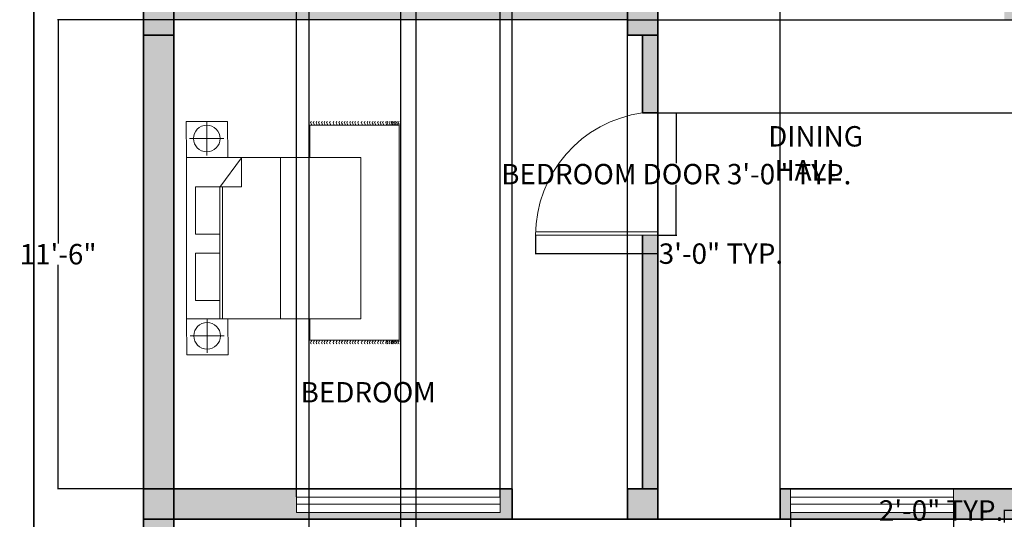
# Model space of a CAD drawing. Units: inches. Extents: x 74 to 548, y 68 to 649.
# Tile 2 of 6: x 79 to 368, y 214 to 361. Entities that reach past the tile are written whole.
import ezdxf

# ---------------------------------------------------------------- set-up
doc = ezdxf.new("R2010")
doc.units = ezdxf.units.IN
doc.header["$MEASUREMENT"] = 0
for name, color, linetype, lineweight in [('A-ANNO-DIMS', 2, 'Continuous', 18), ('A-ANNO-TTLB', 7, 'Continuous', 35), ('A-AREA-IDEN', 7, 'Continuous', 25), ('A-COLS', 7, 'Continuous', 35), ('A-DOOR', 3, 'Continuous', 18), ('A-FURN', 8, 'Continuous', 18), ('A-GLAZ', 4, 'Continuous', 18), ('A-WALL', 7, 'Continuous', 35)]:
    doc.layers.add(name, color=color, linetype=linetype, lineweight=lineweight)
doc.layers.add('A-COLS-PATT', color=11, linetype='Continuous', lineweight=13, true_color=0xf27172)
doc.layers.add('A-WALL-PATT', color=7, linetype='Continuous', lineweight=13, true_color=0xffffff)
doc.styles.get("Standard").update_dxf_attribs({"font": 'arial.ttf'})
doc.dimstyles.get("Standard").update_dxf_attribs({"dimtxt": 6, "dimasz": 0.18, "dimexe": 0.18, "dimexo": 0.0625, "dimgap": 0.09, "dimtad": 0, "dimtih": 1, "dimtoh": 1, "dimdec": 1, "dimzin": 0, "dimdsep": 46, "dimlunit": 3, "dimtxsty": 'Standard', "dimcen": 0.09, "dimadec": 0, "dimazin": 0, "dimtfac": 1, "dimtdec": 1, "dimtofl": 0, "dimtmove": 0, "dimatfit": 3, "dimfxl": 1, "dimtolj": 1, "dimtzin": 0, "dimarcsym": 0})

# ---------------------------------------------------------------- blocks, each defined once
blk = doc.blocks.new('BED-DOUBLE-NIGHTSTANDS')
for p, q in [((-5.03, -1.07), (-5.03, -11.12)), ((53.03, -0.96), (53.03, -11.02)), ((0, -6.09), (-10.05, -6.09)), ((58.05, -5.99), (48, -5.99)), ((38.76, -9.86), (0, -9.86)), ((38.82, -10.68), (0, -10.68)), ((38.76, -9.86), (47.38, -16.22)), ((38.82, -9.86), (38.82, -16.22)), ((38.82, -16.22), (47.38, -16.22)), ((47.43, -27.72), (0, -27.72)), ((-6.27, -62.68), (-6.27, -36.31)), ((-6.27, -36.31), (0.03, -36.31)), ((47.43, -36.31), (56.97, -36.31)), ((56.97, -36.31), (56.97, -62.68)), ((56.97, -62.68), (-6.27, -62.68))]:
    blk.add_line(p, q)
for points in [[(-10.63, -12.29), (0, -12.19), (0, 0), (-10.63, -0.1)], [(47.43, 0), (47.43, -51.32), (0, -51.32), (0, 0)], [(47.43, -12.19), (58.05, -12.08), (58.05, 0.1), (47.43, 0)], [(19.25, -2.7), (19.25, -9.86), (5.36, -9.86), (5.36, -2.7)], [(38.82, -2.7), (38.82, -9.86), (24.92, -9.86), (24.92, -2.7)]]:
    blk.add_lwpolyline(points, close=True)
for centre in [(-5.03, -6.09), (53.03, -5.99)]:
    blk.add_circle(centre, 3.92)
for points, knots in [([(-7.4, -36.85), (-7.3, -36.72), (-7.11, -36.49), (-6.77, -36.72), (-6.49, -36.9), (-6.34, -36.79), (-6.27, -36.74)], [0, 0, 0, 0, 0.400747, 0.791423, 1.067667, 1.29709, 1.29709, 1.29709, 1.29709]), ([(-7.4, -37.62), (-7.3, -37.5), (-7.11, -37.26), (-6.77, -37.5), (-6.49, -37.68), (-6.34, -37.57), (-6.27, -37.52)], [0, 0, 0, 0, 0.400747, 0.791423, 1.067667, 1.29709, 1.29709, 1.29709, 1.29709]), ([(58.08, -36.85), (57.99, -36.72), (57.8, -36.49), (57.45, -36.72), (57.17, -36.9), (57.02, -36.79), (56.96, -36.74)], [0, 0, 0, 0, 0.400747, 0.791423, 1.067667, 1.29709, 1.29709, 1.29709, 1.29709]), ([(58.08, -37.62), (57.99, -37.5), (57.8, -37.26), (57.45, -37.5), (57.17, -37.68), (57.02, -37.57), (56.96, -37.52)], [0, 0, 0, 0, 0.400747, 0.791423, 1.067667, 1.29709, 1.29709, 1.29709, 1.29709]), ([(-7.4, -38.44), (-7.3, -38.32), (-7.11, -38.08), (-6.77, -38.32), (-6.49, -38.49), (-6.34, -38.39), (-6.27, -38.34)], [0, 0, 0, 0, 0.400747, 0.791423, 1.067667, 1.29709, 1.29709, 1.29709, 1.29709]), ([(-7.4, -39.17), (-7.3, -39.05), (-7.11, -38.81), (-6.77, -39.05), (-6.49, -39.22), (-6.34, -39.11), (-6.27, -39.07)], [0, 0, 0, 0, 0.400747, 0.791423, 1.067667, 1.29709, 1.29709, 1.29709, 1.29709]), ([(-7.4, -40.05), (-7.3, -39.93), (-7.11, -39.69), (-6.77, -39.93), (-6.49, -40.1), (-6.34, -40), (-6.27, -39.95)], [0, 0, 0, 0, 0.400747, 0.791423, 1.067667, 1.29709, 1.29709, 1.29709, 1.29709]), ([(-7.4, -40.8), (-7.3, -40.68), (-7.11, -40.44), (-6.77, -40.68), (-6.49, -40.85), (-6.34, -40.75), (-6.27, -40.7)], [0, 0, 0, 0, 0.400747, 0.791423, 1.067667, 1.29709, 1.29709, 1.29709, 1.29709]), ([(58.08, -38.44), (57.99, -38.32), (57.8, -38.08), (57.45, -38.32), (57.17, -38.49), (57.02, -38.39), (56.96, -38.34)], [0, 0, 0, 0, 0.400747, 0.791423, 1.067667, 1.29709, 1.29709, 1.29709, 1.29709]), ([(58.08, -39.17), (57.99, -39.05), (57.8, -38.81), (57.45, -39.05), (57.17, -39.22), (57.02, -39.11), (56.96, -39.07)], [0, 0, 0, 0, 0.400747, 0.791423, 1.067667, 1.29709, 1.29709, 1.29709, 1.29709]), ([(58.08, -40.05), (57.99, -39.93), (57.8, -39.69), (57.45, -39.93), (57.17, -40.1), (57.02, -40), (56.96, -39.95)], [0, 0, 0, 0, 0.400747, 0.791423, 1.067667, 1.29709, 1.29709, 1.29709, 1.29709]), ([(58.08, -40.8), (57.99, -40.68), (57.8, -40.44), (57.45, -40.68), (57.17, -40.85), (57.02, -40.75), (56.96, -40.7)], [0, 0, 0, 0, 0.400747, 0.791423, 1.067667, 1.29709, 1.29709, 1.29709, 1.29709]), ([(-7.4, -41.53), (-7.3, -41.41), (-7.11, -41.17), (-6.77, -41.41), (-6.49, -41.58), (-6.34, -41.48), (-6.27, -41.43)], [0, 0, 0, 0, 0.400747, 0.791423, 1.067667, 1.29709, 1.29709, 1.29709, 1.29709]), ([(-7.4, -42.41), (-7.3, -42.29), (-7.11, -42.05), (-6.77, -42.29), (-6.49, -42.46), (-6.34, -42.36), (-6.27, -42.31)], [0, 0, 0, 0, 0.400747, 0.791423, 1.067667, 1.29709, 1.29709, 1.29709, 1.29709]), ([(-7.4, -43.45), (-7.3, -43.33), (-7.11, -43.09), (-6.77, -43.33), (-6.49, -43.5), (-6.34, -43.39), (-6.27, -43.35)], [0, 0, 0, 0, 0.400747, 0.791423, 1.067667, 1.29709, 1.29709, 1.29709, 1.29709]), ([(58.08, -41.53), (57.99, -41.41), (57.8, -41.17), (57.45, -41.41), (57.17, -41.58), (57.02, -41.48), (56.96, -41.43)], [0, 0, 0, 0, 0.400747, 0.791423, 1.067667, 1.29709, 1.29709, 1.29709, 1.29709]), ([(58.08, -42.41), (57.99, -42.29), (57.8, -42.05), (57.45, -42.29), (57.17, -42.46), (57.02, -42.36), (56.96, -42.31)], [0, 0, 0, 0, 0.400747, 0.791423, 1.067667, 1.29709, 1.29709, 1.29709, 1.29709]), ([(58.08, -43.45), (57.99, -43.33), (57.8, -43.09), (57.45, -43.33), (57.17, -43.5), (57.02, -43.39), (56.96, -43.35)], [0, 0, 0, 0, 0.400747, 0.791423, 1.067667, 1.29709, 1.29709, 1.29709, 1.29709]), ([(-7.4, -44.33), (-7.3, -44.21), (-7.11, -43.97), (-6.77, -44.21), (-6.49, -44.38), (-6.34, -44.28), (-6.27, -44.23)], [0, 0, 0, 0, 0.400747, 0.791423, 1.067667, 1.29709, 1.29709, 1.29709, 1.29709]), ([(-7.4, -45.15), (-7.3, -45.03), (-7.11, -44.79), (-6.77, -45.03), (-6.49, -45.2), (-6.34, -45.09), (-6.27, -45.05)], [0, 0, 0, 0, 0.400747, 0.791423, 1.067667, 1.29709, 1.29709, 1.29709, 1.29709]), ([(-7.4, -45.92), (-7.3, -45.8), (-7.11, -45.56), (-6.77, -45.8), (-6.49, -45.98), (-6.34, -45.87), (-6.27, -45.82)], [0, 0, 0, 0, 0.400747, 0.791423, 1.067667, 1.29709, 1.29709, 1.29709, 1.29709]), ([(58.08, -44.33), (57.99, -44.21), (57.8, -43.97), (57.45, -44.21), (57.17, -44.38), (57.02, -44.28), (56.96, -44.23)], [0, 0, 0, 0, 0.400747, 0.791423, 1.067667, 1.29709, 1.29709, 1.29709, 1.29709]), ([(58.08, -45.15), (57.99, -45.03), (57.8, -44.79), (57.45, -45.03), (57.17, -45.2), (57.02, -45.09), (56.96, -45.05)], [0, 0, 0, 0, 0.400747, 0.791423, 1.067667, 1.29709, 1.29709, 1.29709, 1.29709]), ([(58.08, -45.92), (57.99, -45.8), (57.8, -45.56), (57.45, -45.8), (57.17, -45.98), (57.02, -45.87), (56.96, -45.82)], [0, 0, 0, 0, 0.400747, 0.791423, 1.067667, 1.29709, 1.29709, 1.29709, 1.29709]), ([(-7.4, -46.74), (-7.3, -46.62), (-7.11, -46.38), (-6.77, -46.62), (-6.49, -46.79), (-6.34, -46.69), (-6.27, -46.64)], [0, 0, 0, 0, 0.400747, 0.791423, 1.067667, 1.29709, 1.29709, 1.29709, 1.29709]), ([(-7.4, -47.47), (-7.3, -47.35), (-7.11, -47.11), (-6.77, -47.35), (-6.49, -47.52), (-6.34, -47.41), (-6.27, -47.37)], [0, 0, 0, 0, 0.400747, 0.791423, 1.067667, 1.29709, 1.29709, 1.29709, 1.29709]), ([(-7.4, -48.35), (-7.3, -48.23), (-7.11, -47.99), (-6.77, -48.23), (-6.49, -48.4), (-6.34, -48.3), (-6.27, -48.25)], [0, 0, 0, 0, 0.400747, 0.791423, 1.067667, 1.29709, 1.29709, 1.29709, 1.29709]), ([(-7.4, -49.1), (-7.3, -48.98), (-7.11, -48.74), (-6.77, -48.98), (-6.49, -49.15), (-6.34, -49.05), (-6.27, -49)], [0, 0, 0, 0, 0.400747, 0.791423, 1.067667, 1.29709, 1.29709, 1.29709, 1.29709]), ([(58.08, -46.74), (57.99, -46.62), (57.8, -46.38), (57.45, -46.62), (57.17, -46.79), (57.02, -46.69), (56.96, -46.64)], [0, 0, 0, 0, 0.400747, 0.791423, 1.067667, 1.29709, 1.29709, 1.29709, 1.29709]), ([(58.08, -47.47), (57.99, -47.35), (57.8, -47.11), (57.45, -47.35), (57.17, -47.52), (57.02, -47.41), (56.96, -47.37)], [0, 0, 0, 0, 0.400747, 0.791423, 1.067667, 1.29709, 1.29709, 1.29709, 1.29709]), ([(58.08, -48.35), (57.99, -48.23), (57.8, -47.99), (57.45, -48.23), (57.17, -48.4), (57.02, -48.3), (56.96, -48.25)], [0, 0, 0, 0, 0.400747, 0.791423, 1.067667, 1.29709, 1.29709, 1.29709, 1.29709]), ([(58.08, -49.1), (57.99, -48.98), (57.8, -48.74), (57.45, -48.98), (57.17, -49.15), (57.02, -49.05), (56.96, -49)], [0, 0, 0, 0, 0.400747, 0.791423, 1.067667, 1.29709, 1.29709, 1.29709, 1.29709]), ([(-7.4, -49.83), (-7.3, -49.71), (-7.11, -49.47), (-6.77, -49.71), (-6.49, -49.88), (-6.34, -49.78), (-6.27, -49.73)], [0, 0, 0, 0, 0.400747, 0.791423, 1.067667, 1.29709, 1.29709, 1.29709, 1.29709]), ([(-7.4, -50.71), (-7.3, -50.59), (-7.11, -50.35), (-6.77, -50.59), (-6.49, -50.77), (-6.34, -50.66), (-6.27, -50.61)], [0, 0, 0, 0, 0.400747, 0.791423, 1.067667, 1.29709, 1.29709, 1.29709, 1.29709]), ([(-7.4, -51.75), (-7.3, -51.63), (-7.11, -51.39), (-6.77, -51.63), (-6.49, -51.8), (-6.34, -51.7), (-6.27, -51.65)], [0, 0, 0, 0, 0.400747, 0.791423, 1.067667, 1.29709, 1.29709, 1.29709, 1.29709]), ([(58.08, -49.83), (57.99, -49.71), (57.8, -49.47), (57.45, -49.71), (57.17, -49.88), (57.02, -49.78), (56.96, -49.73)], [0, 0, 0, 0, 0.400747, 0.791423, 1.067667, 1.29709, 1.29709, 1.29709, 1.29709]), ([(58.08, -50.71), (57.99, -50.59), (57.8, -50.35), (57.45, -50.59), (57.17, -50.77), (57.02, -50.66), (56.96, -50.61)], [0, 0, 0, 0, 0.400747, 0.791423, 1.067667, 1.29709, 1.29709, 1.29709, 1.29709]), ([(58.08, -51.75), (57.99, -51.63), (57.8, -51.39), (57.45, -51.63), (57.17, -51.8), (57.02, -51.7), (56.96, -51.65)], [0, 0, 0, 0, 0.400747, 0.791423, 1.067667, 1.29709, 1.29709, 1.29709, 1.29709]), ([(-7.4, -52.63), (-7.3, -52.51), (-7.11, -52.27), (-6.77, -52.51), (-6.49, -52.68), (-6.34, -52.58), (-6.27, -52.53)], [0, 0, 0, 0, 0.400747, 0.791423, 1.067667, 1.29709, 1.29709, 1.29709, 1.29709]), ([(-7.4, -53.45), (-7.3, -53.33), (-7.11, -53.09), (-6.77, -53.33), (-6.49, -53.5), (-6.34, -53.39), (-6.27, -53.35)], [0, 0, 0, 0, 0.400747, 0.791423, 1.067667, 1.29709, 1.29709, 1.29709, 1.29709]), ([(-7.4, -54.14), (-7.3, -54.02), (-7.11, -53.78), (-6.77, -54.02), (-6.49, -54.19), (-6.34, -54.08), (-6.27, -54.04)], [0, 0, 0, 0, 0.400747, 0.791423, 1.067667, 1.29709, 1.29709, 1.29709, 1.29709]), ([(-7.4, -54.95), (-7.3, -54.83), (-7.11, -54.59), (-6.77, -54.83), (-6.49, -55.01), (-6.34, -54.9), (-6.27, -54.85)], [0, 0, 0, 0, 0.400747, 0.791423, 1.067667, 1.29709, 1.29709, 1.29709, 1.29709]), ([(58.08, -52.63), (57.99, -52.51), (57.8, -52.27), (57.45, -52.51), (57.17, -52.68), (57.02, -52.58), (56.96, -52.53)], [0, 0, 0, 0, 0.400747, 0.791423, 1.067667, 1.29709, 1.29709, 1.29709, 1.29709]), ([(58.08, -53.45), (57.99, -53.33), (57.8, -53.09), (57.45, -53.33), (57.17, -53.5), (57.02, -53.39), (56.96, -53.35)], [0, 0, 0, 0, 0.400747, 0.791423, 1.067667, 1.29709, 1.29709, 1.29709, 1.29709]), ([(58.08, -54.14), (57.99, -54.02), (57.8, -53.78), (57.45, -54.02), (57.17, -54.19), (57.02, -54.08), (56.96, -54.04)], [0, 0, 0, 0, 0.400747, 0.791423, 1.067667, 1.29709, 1.29709, 1.29709, 1.29709]), ([(58.08, -54.95), (57.99, -54.83), (57.8, -54.59), (57.45, -54.83), (57.17, -55.01), (57.02, -54.9), (56.96, -54.85)], [0, 0, 0, 0, 0.400747, 0.791423, 1.067667, 1.29709, 1.29709, 1.29709, 1.29709]), ([(-7.4, -55.68), (-7.3, -55.56), (-7.11, -55.32), (-6.77, -55.56), (-6.49, -55.73), (-6.34, -55.63), (-6.27, -55.58)], [0, 0, 0, 0, 0.400747, 0.791423, 1.067667, 1.29709, 1.29709, 1.29709, 1.29709]), ([(-7.4, -56.56), (-7.3, -56.44), (-7.11, -56.2), (-6.77, -56.44), (-6.49, -56.62), (-6.34, -56.51), (-6.27, -56.46)], [0, 0, 0, 0, 0.400747, 0.791423, 1.067667, 1.29709, 1.29709, 1.29709, 1.29709]), ([(-7.4, -57.32), (-7.3, -57.2), (-7.11, -56.96), (-6.77, -57.2), (-6.49, -57.37), (-6.34, -57.26), (-6.27, -57.21)], [0, 0, 0, 0, 0.400747, 0.791423, 1.067667, 1.29709, 1.29709, 1.29709, 1.29709]), ([(-7.4, -58.04), (-7.3, -57.92), (-7.11, -57.68), (-6.77, -57.92), (-6.49, -58.1), (-6.34, -57.99), (-6.27, -57.94)], [0, 0, 0, 0, 0.400747, 0.791423, 1.067667, 1.29709, 1.29709, 1.29709, 1.29709]), ([(58.08, -55.68), (57.99, -55.56), (57.8, -55.32), (57.45, -55.56), (57.17, -55.73), (57.02, -55.63), (56.96, -55.58)], [0, 0, 0, 0, 0.400747, 0.791423, 1.067667, 1.29709, 1.29709, 1.29709, 1.29709]), ([(58.08, -56.56), (57.99, -56.44), (57.8, -56.2), (57.45, -56.44), (57.17, -56.62), (57.02, -56.51), (56.96, -56.46)], [0, 0, 0, 0, 0.400747, 0.791423, 1.067667, 1.29709, 1.29709, 1.29709, 1.29709]), ([(58.08, -57.32), (57.99, -57.2), (57.8, -56.96), (57.45, -57.2), (57.17, -57.37), (57.02, -57.26), (56.96, -57.21)], [0, 0, 0, 0, 0.400747, 0.791423, 1.067667, 1.29709, 1.29709, 1.29709, 1.29709]), ([(58.08, -58.04), (57.99, -57.92), (57.8, -57.68), (57.45, -57.92), (57.18, -58.09), (57.03, -57.99), (56.97, -57.95)], [0, 0, 0, 0, 0.400747, 0.791423, 1.067667, 1.283686, 1.283686, 1.283686, 1.283686]), ([(-7.4, -58.93), (-7.3, -58.81), (-7.11, -58.57), (-6.77, -58.81), (-6.49, -58.98), (-6.34, -58.87), (-6.27, -58.82)], [0, 0, 0, 0, 0.400747, 0.791423, 1.067667, 1.29709, 1.29709, 1.29709, 1.29709]), ([(-7.4, -59.36), (-7.3, -59.23), (-7.11, -58.98), (-6.77, -59.24), (-6.49, -59.41), (-6.34, -59.3), (-6.27, -59.25)], [0, 0, 0, 0, 0.407265, 0.802015, 1.07826, 1.307683, 1.307683, 1.307683, 1.307683]), ([(-7.4, -59.92), (-7.3, -59.8), (-7.11, -59.56), (-6.77, -59.8), (-6.49, -59.97), (-6.34, -59.87), (-6.27, -59.82)], [0, 0, 0, 0, 0.400747, 0.791423, 1.067667, 1.29709, 1.29709, 1.29709, 1.29709]), ([(-7.4, -60.5), (-7.3, -60.38), (-7.11, -60.14), (-6.77, -60.38), (-6.49, -60.55), (-6.34, -60.44), (-6.27, -60.39)], [0, 0, 0, 0, 0.400747, 0.791423, 1.067667, 1.29709, 1.29709, 1.29709, 1.29709]), ([(-7.4, -60.81), (-7.3, -60.68), (-7.11, -60.44), (-6.77, -60.68), (-6.49, -60.86), (-6.34, -60.75), (-6.27, -60.7)], [0, 0, 0, 0, 0.400747, 0.791423, 1.067667, 1.29709, 1.29709, 1.29709, 1.29709]), ([(58.08, -58.93), (57.99, -58.81), (57.8, -58.57), (57.45, -58.81), (57.18, -58.98), (57.03, -58.88), (56.97, -58.83)], [0, 0, 0, 0, 0.400747, 0.791423, 1.067667, 1.283686, 1.283686, 1.283686, 1.283686]), ([(58.08, -59.36), (57.99, -59.23), (57.8, -58.99), (57.45, -59.24), (57.18, -59.41), (57.03, -59.31), (56.97, -59.26)], [0, 0, 0, 0, 0.402903, 0.794912, 1.071156, 1.287177, 1.287177, 1.287177, 1.287177]), ([(58.08, -59.95), (57.99, -59.83), (57.8, -59.59), (57.45, -59.83), (57.18, -60), (57.03, -59.9), (56.97, -59.86)], [0, 0, 0, 0, 0.400747, 0.791423, 1.067667, 1.283686, 1.283686, 1.283686, 1.283686]), ([(58.08, -60.52), (57.99, -60.4), (57.8, -60.16), (57.45, -60.4), (57.18, -60.57), (57.03, -60.47), (56.97, -60.43)], [0, 0, 0, 0, 0.400747, 0.791423, 1.067667, 1.283686, 1.283686, 1.283686, 1.283686]), ([(58.08, -60.83), (57.99, -60.71), (57.8, -60.47), (57.45, -60.71), (57.18, -60.88), (57.03, -60.78), (56.97, -60.74)], [0, 0, 0, 0, 0.400747, 0.791423, 1.067667, 1.283686, 1.283686, 1.283686, 1.283686]), ([(-7.4, -61.22), (-7.3, -61.1), (-7.11, -60.86), (-6.77, -61.1), (-6.49, -61.28), (-6.34, -61.17), (-6.27, -61.12)], [0, 0, 0, 0, 0.400747, 0.791423, 1.067667, 1.29709, 1.29709, 1.29709, 1.29709]), ([(-7.4, -61.62), (-7.3, -61.5), (-7.11, -61.26), (-6.77, -61.5), (-6.49, -61.67), (-6.34, -61.57), (-6.27, -61.52)], [0, 0, 0, 0, 0.400747, 0.791423, 1.067667, 1.29709, 1.29709, 1.29709, 1.29709]), ([(-7.4, -62.11), (-7.3, -61.99), (-7.11, -61.75), (-6.77, -61.99), (-6.49, -62.16), (-6.34, -62.05), (-6.27, -62)], [0, 0, 0, 0, 0.400747, 0.791423, 1.067667, 1.29709, 1.29709, 1.29709, 1.29709]), ([(-7.4, -62.61), (-7.3, -62.49), (-7.11, -62.25), (-6.77, -62.49), (-6.49, -62.66), (-6.34, -62.55), (-6.27, -62.51)], [0, 0, 0, 0, 0.400747, 0.791423, 1.067667, 1.29709, 1.29709, 1.29709, 1.29709]), ([(58.08, -61.25), (57.99, -61.13), (57.8, -60.89), (57.45, -61.13), (57.17, -61.3), (57.02, -61.2), (56.96, -61.15)], [0, 0, 0, 0, 0.400747, 0.791423, 1.067667, 1.29709, 1.29709, 1.29709, 1.29709]), ([(58.08, -61.65), (57.99, -61.53), (57.8, -61.29), (57.45, -61.53), (57.17, -61.7), (57.02, -61.6), (56.96, -61.55)], [0, 0, 0, 0, 0.400747, 0.791423, 1.067667, 1.29709, 1.29709, 1.29709, 1.29709]), ([(58.08, -62.13), (57.99, -62.01), (57.8, -61.77), (57.45, -62.01), (57.17, -62.19), (57.02, -62.08), (56.96, -62.03)], [0, 0, 0, 0, 0.400747, 0.791423, 1.067667, 1.29709, 1.29709, 1.29709, 1.29709]), ([(58.08, -62.61), (57.99, -62.49), (57.8, -62.25), (57.45, -62.49), (57.17, -62.66), (57.02, -62.55), (56.96, -62.51)], [0, 0, 0, 0, 0.400747, 0.791423, 1.067667, 1.29709, 1.29709, 1.29709, 1.29709])]:
    blk.add_open_spline(points, degree=3, knots=knots)
blk = doc.blocks.new('DOOR-SWING-36IN')
for p, q in [((0, 0), (0, 36)), ((-36, 1), (0, 1)), ((0, 0), (-36, 0))]:
    blk.add_line(p, q)
blk.add_arc((0.32, 0), 36.32, 97.6281, 180)
blk = doc.blocks.new('*D14')
at = {"layer": 'A-ANNO-DIMS', "color": 0, "lineweight": -2, "transparency": 16777216}
for p, q in [((266.52, 333.81), (272.04, 333.81)), ((271.86, 333.63), (271.86, 319.01)), ((271.86, 297.99), (271.86, 312.61)), ((266.52, 297.81), (272.04, 297.81))]:
    blk.add_line(p, q, dxfattribs=at)
at = {"layer": 'A-ANNO-DIMS', "color": 0, "transparency": 16777216}
for points in [[(271.83, 333.63), (271.89, 333.63), (271.86, 333.81)], [(271.83, 297.99), (271.89, 297.99), (271.86, 297.81)]]:
    blk.add_solid(points, dxfattribs=at)
at = {"layer": 'Defpoints', "color": 0, "transparency": 16777216}
for p in [(266.46, 333.81), (271.86, 333.81), (266.46, 297.81)]:
    blk.add_point(p, dxfattribs=at)
at = {"layer": 'A-ANNO-DIMS', "color": 0, "transparency": 16777216, "insert": (271.86, 315.81), "char_height": 6, "attachment_point": 5}
blk.add_mtext('\\A1;BEDROOM DOOR 3\'-0" TYP.', dxfattribs=at)
blk = doc.blocks.new('*D15')
at = {"layer": 'A-ANNO-DIMS', "color": 0, "lineweight": -2, "transparency": 16777216}
for p, q in [((230.46, 297.75), (230.46, 292.23)), ((266.46, 297.75), (266.46, 292.23)), ((230.64, 292.41), (266.28, 292.41)), ((266.46, 292.41), (266.64, 292.41))]:
    blk.add_line(p, q, dxfattribs=at)
at = {"layer": 'A-ANNO-DIMS', "color": 0, "transparency": 16777216}
for points in [[(230.64, 292.44), (230.64, 292.38), (230.46, 292.41)], [(266.28, 292.44), (266.28, 292.38), (266.46, 292.41)]]:
    blk.add_solid(points, dxfattribs=at)
at = {"layer": 'Defpoints', "color": 0, "transparency": 16777216}
for p in [(230.46, 297.81), (266.46, 297.81), (266.46, 292.41)]:
    blk.add_point(p, dxfattribs=at)
at = {"layer": 'A-ANNO-DIMS', "color": 0, "transparency": 16777216, "insert": (285.02, 292.41), "char_height": 6, "attachment_point": 5}
blk.add_mtext('\\A1;3\'-0" TYP.', dxfattribs=at)
blk = doc.blocks.new('*D16')
at = {"layer": 'A-ANNO-DIMS', "color": 0, "lineweight": -2, "transparency": 16777216}
for p, q in [((392.52, 213.24), (396.24, 213.24)), ((396.06, 213.06), (396.06, 204.44)), ((396.06, 189.42), (396.06, 198.05)), ((392.52, 189.24), (396.24, 189.24))]:
    blk.add_line(p, q, dxfattribs=at)
at = {"layer": 'A-ANNO-DIMS', "color": 0, "transparency": 16777216}
for points in [[(396.03, 213.06), (396.09, 213.06), (396.06, 213.24)], [(396.03, 189.42), (396.09, 189.42), (396.06, 189.24)]]:
    blk.add_solid(points, dxfattribs=at)
at = {"layer": 'Defpoints', "color": 0, "transparency": 16777216}
for p in [(392.46, 213.24), (396.06, 213.24), (392.46, 189.24)]:
    blk.add_point(p, dxfattribs=at)
at = {"layer": 'A-ANNO-DIMS', "color": 0, "transparency": 16777216, "insert": (396.06, 201.24), "char_height": 6, "attachment_point": 5}
blk.add_mtext('\\A1;ROOM DOOR 2\'-0" TYP.', dxfattribs=at)
blk = doc.blocks.new('*D17')
at = {"layer": 'A-ANNO-DIMS', "color": 0, "lineweight": -2, "transparency": 16777216}
for p, q in [((368.46, 216.84), (368.28, 216.84)), ((368.46, 213.31), (368.46, 217.02)), ((392.28, 216.84), (368.64, 216.84)), ((392.46, 213.31), (392.46, 217.02))]:
    blk.add_line(p, q, dxfattribs=at)
at = {"layer": 'A-ANNO-DIMS', "color": 0, "transparency": 16777216}
for points in [[(368.64, 216.87), (368.64, 216.81), (368.46, 216.84)], [(392.28, 216.87), (392.28, 216.81), (392.46, 216.84)]]:
    blk.add_solid(points, dxfattribs=at)
at = {"layer": 'Defpoints', "color": 0, "transparency": 16777216}
for p in [(368.46, 216.84), (368.46, 213.24), (392.46, 213.24)]:
    blk.add_point(p, dxfattribs=at)
at = {"layer": 'A-ANNO-DIMS', "color": 0, "transparency": 16777216, "insert": (349.85, 216.84), "char_height": 6, "attachment_point": 5}
blk.add_mtext('\\A1;2\'-0" TYP.', dxfattribs=at)
blk = doc.blocks.new('*D19')
at = {"layer": 'A-ANNO-DIMS', "color": 0, "lineweight": -2, "transparency": 16777216}
for p, q in [((123.96, 361.31), (123.96, 609.52)), ((124.14, 609.34), (149.27, 609.34)), ((190.53, 609.34), (165.4, 609.34)), ((190.71, 365.81), (190.71, 609.52))]:
    blk.add_line(p, q, dxfattribs=at)
at = {"layer": 'A-ANNO-DIMS', "color": 0, "transparency": 16777216}
for points in [[(124.14, 609.37), (124.14, 609.31), (123.96, 609.34)], [(190.53, 609.37), (190.53, 609.31), (190.71, 609.34)]]:
    blk.add_solid(points, dxfattribs=at)
at = {"layer": 'Defpoints', "color": 0, "transparency": 16777216}
for p in [(190.71, 609.34), (190.71, 365.74), (123.96, 361.24)]:
    blk.add_point(p, dxfattribs=at)
at = {"layer": 'A-ANNO-DIMS', "color": 0, "transparency": 16777216, "insert": (157.34, 609.34), "char_height": 6, "attachment_point": 5}
blk.add_mtext('\\A1;5\'-7"', dxfattribs=at)
blk = doc.blocks.new('*D23')
at = {"layer": 'A-ANNO-DIMS', "color": 0, "lineweight": -2, "transparency": 16777216}
for p, q in [((257.4, 361.24), (89.68, 361.24)), ((89.86, 361.06), (89.86, 295.4)), ((89.86, 223.42), (89.86, 289.09)), ((223.52, 223.24), (89.68, 223.24))]:
    blk.add_line(p, q, dxfattribs=at)
at = {"layer": 'A-ANNO-DIMS', "color": 0, "transparency": 16777216}
for points in [[(89.83, 361.06), (89.89, 361.06), (89.86, 361.24)], [(89.83, 223.42), (89.89, 223.42), (89.86, 223.24)]]:
    blk.add_solid(points, dxfattribs=at)
at = {"layer": 'Defpoints', "color": 0, "transparency": 16777216}
for p in [(89.86, 361.24), (257.46, 361.24), (223.59, 223.24)]:
    blk.add_point(p, dxfattribs=at)
at = {"layer": 'A-ANNO-DIMS', "color": 0, "transparency": 16777216, "insert": (89.86, 292.24), "char_height": 6, "attachment_point": 5}
blk.add_mtext('\\A1;11\'-6"', dxfattribs=at)
blk = doc.blocks.new('*D30')
at = {"layer": 'A-ANNO-DIMS', "color": 0, "lineweight": -2, "transparency": 16777216}
for p, q in [((160.05, 220.81), (160.05, 609.52)), ((160.23, 609.34), (181.98, 609.34)), ((219.87, 609.34), (198.11, 609.34)), ((220.05, 220.81), (220.05, 609.52))]:
    blk.add_line(p, q, dxfattribs=at)
at = {"layer": 'A-ANNO-DIMS', "color": 0, "transparency": 16777216}
for points in [[(160.23, 609.37), (160.23, 609.31), (160.05, 609.34)], [(219.87, 609.37), (219.87, 609.31), (220.05, 609.34)]]:
    blk.add_solid(points, dxfattribs=at)
at = {"layer": 'Defpoints', "color": 0, "transparency": 16777216}
for p in [(220.05, 609.34), (160.05, 220.74), (220.05, 220.74)]:
    blk.add_point(p, dxfattribs=at)
at = {"layer": 'A-ANNO-DIMS', "color": 0, "transparency": 16777216, "insert": (190.05, 609.34), "char_height": 6, "attachment_point": 5}
blk.add_mtext('\\A1;5\'-0"', dxfattribs=at)
blk = doc.blocks.new('*D31')
at = {"layer": 'A-ANNO-DIMS', "color": 0, "lineweight": -2, "transparency": 16777216}
for p, q in [((305.46, 216.18), (305.46, 87.96)), ((353.46, 216.18), (353.46, 87.96)), ((305.64, 88.14), (321.28, 88.14)), ((353.28, 88.14), (337.65, 88.14))]:
    blk.add_line(p, q, dxfattribs=at)
at = {"layer": 'A-ANNO-DIMS', "color": 0, "transparency": 16777216}
for points in [[(305.64, 88.17), (305.64, 88.11), (305.46, 88.14)], [(353.28, 88.17), (353.28, 88.11), (353.46, 88.14)]]:
    blk.add_solid(points, dxfattribs=at)
at = {"layer": 'Defpoints', "color": 0, "transparency": 16777216}
for p in [(305.46, 216.24), (353.46, 216.24), (353.46, 88.14)]:
    blk.add_point(p, dxfattribs=at)
at = {"layer": 'A-ANNO-DIMS', "color": 0, "transparency": 16777216, "insert": (329.46, 88.14), "char_height": 6, "attachment_point": 5}
blk.add_mtext('\\A1;4\'-0"', dxfattribs=at)
blk = doc.blocks.new('*D35')
at = {"layer": 'A-ANNO-DIMS', "color": 0, "lineweight": -2, "transparency": 16777216}
for p, q in [((190.71, 365.68), (190.71, 87.96)), ((195.21, 365.68), (195.21, 87.96)), ((190.89, 88.14), (195.03, 88.14)), ((195.21, 88.14), (195.39, 88.14))]:
    blk.add_line(p, q, dxfattribs=at)
at = {"layer": 'A-ANNO-DIMS', "color": 0, "transparency": 16777216}
for points in [[(190.89, 88.17), (190.89, 88.11), (190.71, 88.14)], [(195.03, 88.17), (195.03, 88.11), (195.21, 88.14)]]:
    blk.add_solid(points, dxfattribs=at)
at = {"layer": 'Defpoints', "color": 0, "transparency": 16777216}
for p in [(190.71, 365.74), (195.21, 365.74), (195.21, 88.14)]:
    blk.add_point(p, dxfattribs=at)
at = {"layer": 'A-ANNO-DIMS', "color": 0, "transparency": 16777216, "insert": (210.45, 88.14), "char_height": 6, "attachment_point": 5}
blk.add_mtext('\\A1;0\'-4 1/2"', dxfattribs=at)
blk = doc.blocks.new('*D36')
at = {"layer": 'A-ANNO-DIMS', "color": 0, "lineweight": -2, "transparency": 16777216}
for p, q in [((266.46, 223.31), (266.46, 609.52)), ((266.64, 609.34), (276.4, 609.34)), ((302.28, 609.34), (292.52, 609.34)), ((302.46, 223.31), (302.46, 609.52))]:
    blk.add_line(p, q, dxfattribs=at)
at = {"layer": 'A-ANNO-DIMS', "color": 0, "transparency": 16777216}
for points in [[(266.64, 609.37), (266.64, 609.31), (266.46, 609.34)], [(302.28, 609.37), (302.28, 609.31), (302.46, 609.34)]]:
    blk.add_solid(points, dxfattribs=at)
at = {"layer": 'Defpoints', "color": 0, "transparency": 16777216}
for p in [(302.46, 609.34), (266.46, 223.24), (302.46, 223.24)]:
    blk.add_point(p, dxfattribs=at)
at = {"layer": 'A-ANNO-DIMS', "color": 0, "transparency": 16777216, "insert": (284.46, 609.34), "char_height": 6, "attachment_point": 5}
blk.add_mtext('\\A1;3\'-0"', dxfattribs=at)
blk = doc.blocks.new('*D37')
at = {"layer": 'A-ANNO-DIMS', "color": 0, "lineweight": -2, "transparency": 16777216}
for p, q in [((266.46, 297.87), (266.46, 609.52)), ((266.64, 609.34), (322.83, 609.34)), ((399.25, 609.34), (343.06, 609.34)), ((399.43, 299.06), (399.43, 609.52))]:
    blk.add_line(p, q, dxfattribs=at)
at = {"layer": 'A-ANNO-DIMS', "color": 0, "transparency": 16777216}
for points in [[(266.64, 609.37), (266.64, 609.31), (266.46, 609.34)], [(399.25, 609.37), (399.25, 609.31), (399.43, 609.34)]]:
    blk.add_solid(points, dxfattribs=at)
at = {"layer": 'Defpoints', "color": 0, "transparency": 16777216}
for p in [(399.43, 609.34), (399.43, 298.99), (266.46, 297.81)]:
    blk.add_point(p, dxfattribs=at)
at = {"layer": 'A-ANNO-DIMS', "color": 0, "transparency": 16777216, "insert": (332.94, 609.34), "char_height": 6, "attachment_point": 5}
blk.add_mtext('\\A1;11\'-1"', dxfattribs=at)
blk = doc.blocks.new('*D41')
at = {"layer": 'A-ANNO-DIMS', "color": 0, "lineweight": -2, "transparency": 16777216}
for p, q in [((257.52, 361.24), (497.24, 361.24)), ((497.06, 361.06), (497.06, 350.72)), ((497.06, 333.99), (497.06, 344.33)), ((262.02, 333.81), (497.24, 333.81))]:
    blk.add_line(p, q, dxfattribs=at)
at = {"layer": 'A-ANNO-DIMS', "color": 0, "transparency": 16777216}
for points in [[(497.03, 361.06), (497.09, 361.06), (497.06, 361.24)], [(497.03, 333.99), (497.09, 333.99), (497.06, 333.81)]]:
    blk.add_solid(points, dxfattribs=at)
at = {"layer": 'Defpoints', "color": 0, "transparency": 16777216}
for p in [(257.46, 361.24), (497.06, 361.24), (261.96, 333.81)]:
    blk.add_point(p, dxfattribs=at)
at = {"layer": 'A-ANNO-DIMS', "color": 0, "transparency": 16777216, "insert": (497.06, 347.53), "char_height": 6, "attachment_point": 5}
blk.add_mtext('\\A1;2\'-3 1/2"', dxfattribs=at)
blk = doc.blocks.new('*D42')
at = {"layer": 'A-ANNO-DIMS', "color": 0, "lineweight": -2, "transparency": 16777216}
for p, q in [((223.59, 223.31), (223.59, 609.52)), ((223.77, 609.34), (230.08, 609.34)), ((257.28, 609.34), (250.97, 609.34)), ((257.46, 223.31), (257.46, 609.52))]:
    blk.add_line(p, q, dxfattribs=at)
at = {"layer": 'A-ANNO-DIMS', "color": 0, "transparency": 16777216}
for points in [[(223.77, 609.37), (223.77, 609.31), (223.59, 609.34)], [(257.28, 609.37), (257.28, 609.31), (257.46, 609.34)]]:
    blk.add_solid(points, dxfattribs=at)
at = {"layer": 'Defpoints', "color": 0, "transparency": 16777216}
for p in [(257.46, 609.34), (223.59, 223.24), (257.46, 223.24)]:
    blk.add_point(p, dxfattribs=at)
at = {"layer": 'A-ANNO-DIMS', "color": 0, "transparency": 16777216, "insert": (240.52, 609.34), "char_height": 6, "attachment_point": 5}
blk.add_mtext('\\A1;2\'-10"', dxfattribs=at)
blk = doc.blocks.new('*D44')
at = {"layer": 'A-ANNO-DIMS', "color": 0, "lineweight": -2, "transparency": 16777216}
for p, q in [((163.71, 448.18), (163.71, 87.96)), ((123.96, 439.18), (123.96, 87.96)), ((124.14, 88.14), (135.77, 88.14)), ((163.53, 88.14), (151.9, 88.14))]:
    blk.add_line(p, q, dxfattribs=at)
at = {"layer": 'A-ANNO-DIMS', "color": 0, "transparency": 16777216}
for points in [[(124.14, 88.17), (124.14, 88.11), (123.96, 88.14)], [(163.53, 88.17), (163.53, 88.11), (163.71, 88.14)]]:
    blk.add_solid(points, dxfattribs=at)
at = {"layer": 'Defpoints', "color": 0, "transparency": 16777216}
for p in [(163.71, 448.24), (123.96, 439.24), (163.71, 88.14)]:
    blk.add_point(p, dxfattribs=at)
at = {"layer": 'A-ANNO-DIMS', "color": 0, "transparency": 16777216, "insert": (143.84, 88.14), "char_height": 6, "attachment_point": 5}
blk.add_mtext('\\A1;3\'-4"', dxfattribs=at)

msp = doc.modelspace()

# ---------------------------------------------------------------- hatches: boundary and pattern name
at = {"layer": 'A-COLS-PATT'}
h = msp.add_hatch(color=256, dxfattribs=at)
h.dxf.hatch_style = 1
h.paths.add_polyline_path([(123.96, 584.24), (114.96, 584.24), (114.96, 575.24), (123.96, 575.24)])
h.paths.add_polyline_path([(266.46, 584.24), (257.46, 584.24), (257.46, 575.24), (266.46, 575.24)])
h.paths.add_polyline_path([(329.46, 584.24), (320.46, 584.24), (320.46, 575.24), (329.46, 575.24)])
h.paths.add_polyline_path([(471.96, 584.24), (462.96, 584.24), (462.96, 575.24), (471.96, 575.24)])
h.paths.add_polyline_path([(123.96, 448.24), (114.96, 448.24), (114.96, 439.24), (123.96, 439.24)])
h.paths.add_polyline_path([(266.46, 448.24), (261.96, 448.24), (257.46, 448.24), (257.46, 439.24), (266.46, 439.24)])
h.paths.add_polyline_path([(329.46, 448.24), (320.46, 448.24), (320.46, 439.24), (329.46, 439.24)])
h.paths.add_polyline_path([(471.96, 448.24), (462.96, 448.24), (462.96, 439.24), (471.96, 439.24)])
h.paths.add_polyline_path([(123.96, 365.74), (114.96, 365.74), (114.96, 356.74), (123.96, 356.74)])
h.paths.add_polyline_path([(266.46, 365.74), (257.46, 365.74), (257.46, 356.74), (266.46, 356.74)])
h.paths.add_polyline_path([(123.96, 223.24), (114.96, 223.24), (114.96, 214.24), (123.96, 214.24)])
h.paths.add_polyline_path([(266.46, 223.24), (257.46, 223.24), (257.46, 214.24), (266.46, 214.24)])
h.paths.add_polyline_path([(123.96, 142.24), (114.96, 142.24), (114.96, 133.24), (123.96, 133.24)])
h.paths.add_polyline_path([(263.89, 142.24), (254.89, 142.24), (254.89, 133.24), (263.89, 133.24)])
h.paths.add_polyline_path([(471.96, 142.24), (462.96, 142.24), (462.96, 133.24), (471.96, 133.24)])
h.paths.add_polyline_path([(377.46, 142.24), (368.46, 142.24), (368.46, 133.24), (377.46, 133.24)])
h.paths.add_polyline_path([(377.46, 223.24), (368.46, 223.24), (368.46, 214.24), (377.46, 214.24)])
h.paths.add_polyline_path([(471.96, 223.24), (462.96, 223.24), (462.96, 214.24), (471.96, 214.24)])
h.paths.add_polyline_path([(471.96, 298.99), (462.96, 298.99), (462.96, 289.99), (471.96, 289.99)])
h.paths.add_polyline_path([(471.96, 365.74), (462.96, 365.74), (462.96, 356.74), (471.96, 356.74)])
at = {"layer": 'A-WALL-PATT'}
h = msp.add_hatch(color=256, dxfattribs=at)
h.dxf.hatch_style = 1
h.paths.add_polyline_path([(123.96, 356.74), (114.96, 356.74), (114.96, 223.24), (123.96, 223.24)])
h.paths.add_polyline_path([(123.96, 439.24), (114.96, 439.24), (114.96, 365.74), (123.96, 365.74)])
h.paths.add_polyline_path([(123.96, 575.24), (114.96, 575.24), (114.96, 448.24), (123.96, 448.24)])
h.paths.add_polyline_path([(257.46, 584.24), (123.96, 584.24), (123.96, 575.24), (257.46, 575.24)])
h.paths.add_polyline_path([(266.46, 575.24), (261.96, 575.24), (261.96, 490.24), (266.46, 490.24)])
h.paths.add_polyline_path([(266.46, 454.24), (261.96, 454.24), (261.96, 448.24), (266.46, 448.24)])
h.paths.add_polyline_path([(257.46, 448.24), (187.71, 448.24), (187.71, 443.74), (190.71, 443.74), (190.71, 365.74), (123.96, 365.74), (123.96, 361.24), (257.46, 361.24), (257.46, 365.74), (195.21, 365.74), (195.21, 443.74), (257.46, 443.74)])
h.paths.add_polyline_path([(163.71, 448.24), (123.96, 448.24), (123.96, 443.74), (163.71, 443.74)], flags=17)
h.paths.add_polyline_path([(223.59, 223.24), (220.05, 223.24), (220.05, 216.24), (160.05, 216.24), (160.05, 223.24), (123.96, 223.24), (123.96, 214.24), (159.96, 214.24), (223.59, 214.24)])
h.paths.add_polyline_path([(123.96, 214.24), (114.96, 214.24), (114.96, 142.24), (123.96, 142.24)])
h.paths.add_polyline_path([(254.89, 142.24), (123.96, 142.24), (123.96, 133.24), (254.89, 133.24)])
h.paths.add_polyline_path([(462.96, 142.24), (377.46, 142.24), (377.46, 133.24), (462.96, 133.24)])
h.paths.add_polyline_path([(372.96, 189.24), (368.46, 189.24), (368.46, 142.24), (372.96, 142.24)])
h.paths.add_polyline_path([(471.96, 214.24), (462.96, 214.24), (462.96, 142.24), (471.96, 142.24)])
h.paths.add_polyline_path([(462.96, 223.24), (403.93, 223.24), (403.93, 294.49), (409.93, 294.49), (409.93, 298.99), (403.93, 298.99), (399.43, 298.99), (399.43, 223.24), (377.46, 223.24), (377.46, 214.24), (462.96, 214.24)])
h.paths.add_polyline_path([(368.46, 223.24), (353.46, 223.24), (353.46, 216.24), (305.46, 216.24), (305.46, 223.24), (302.46, 223.24), (302.46, 214.24), (368.46, 214.24)])
h.paths.add_polyline_path([(471.96, 289.99), (462.96, 289.99), (462.96, 223.24), (471.96, 223.24)])
h.paths.add_polyline_path([(462.96, 298.99), (433.93, 298.99), (433.93, 294.49), (462.96, 294.49)], flags=0)
h.paths.add_polyline_path([(471.96, 356.74), (462.96, 356.74), (462.96, 298.99), (471.96, 298.99)])
h.paths.add_polyline_path([(462.96, 365.74), (403.93, 365.74), (403.93, 361.24), (462.96, 361.24)], flags=17)
h.paths.add_polyline_path([(471.96, 439.24), (462.96, 439.24), (462.96, 365.74), (471.96, 365.74)])
h.paths.add_polyline_path([(462.96, 448.24), (329.46, 448.24), (329.46, 439.24), (368.46, 439.24), (368.46, 361.24), (372.96, 361.24), (372.96, 443.74), (462.96, 443.74)])
h.paths.add_polyline_path([(324.96, 454.24), (320.46, 454.24), (320.46, 448.24), (324.96, 448.24)])
h.paths.add_polyline_path([(471.96, 575.24), (462.96, 575.24), (462.96, 448.24), (471.96, 448.24)])
h.paths.add_polyline_path([(462.96, 584.24), (329.46, 584.24), (329.46, 575.24), (462.96, 575.24)])
h.paths.add_polyline_path([(320.46, 584.24), (266.46, 584.24), (266.46, 575.24), (320.46, 575.24)])
h.paths.add_polyline_path([(324.96, 575.24), (320.46, 575.24), (320.46, 490.24), (324.96, 490.24)])
h.paths.add_polyline_path([(266.46, 405.58), (257.46, 405.58), (257.46, 365.74), (266.46, 365.74)])
h.paths.add_polyline_path([(266.46, 356.74), (261.96, 356.74), (261.96, 333.81), (266.46, 333.81)])
h.paths.add_polyline_path([(266.46, 297.81), (261.96, 297.81), (261.96, 223.24), (266.46, 223.24)])

# ---------------------------------------------------------------- linework, layer by layer
at = {"layer": 'A-ANNO-TTLB'}
msp.add_lwpolyline([(82.75, 649.38), (548.44, 649.38), (548.44, 68.13), (82.75, 68.13)], close=True, dxfattribs=at)
at = {"layer": 'A-COLS'}
for p, q in [((257.46, 365.74), (257.46, 356.74)), ((114.96, 356.74), (123.96, 356.74)), ((257.46, 356.74), (266.46, 356.74)), ((257.46, 223.24), (257.46, 214.24)), ((257.46, 223.24), (266.46, 223.24))]:
    msp.add_line(p, q, dxfattribs=at)
at = {"layer": 'A-DOOR'}
msp.add_line((230.46, 297.81), (266.46, 297.81), dxfattribs=at)
at = {"layer": 'A-GLAZ'}
for p, q in [((160.05, 216.24), (160.05, 223.24)), ((220.05, 223.24), (220.05, 216.24)), ((305.46, 223.24), (305.46, 216.24)), ((353.46, 216.24), (353.46, 223.24)), ((160.05, 220.74), (220.05, 220.74)), ((305.46, 220.74), (353.46, 220.74)), ((220.05, 218.74), (160.05, 218.74)), ((305.46, 218.74), (353.46, 218.74)), ((220.05, 216.24), (160.05, 216.24)), ((305.46, 216.24), (353.46, 216.24))]:
    msp.add_line(p, q, dxfattribs=at)
at = {"layer": 'A-WALL'}
for p, q in [((114.96, 584.24), (114.96, 133.24)), ((123.96, 584.24), (123.96, 133.24)), ((266.46, 584.24), (266.46, 214.24)), ((261.96, 356.74), (261.96, 333.81)), ((266.46, 333.81), (261.96, 333.81)), ((261.96, 297.81), (261.96, 223.24)), ((114.96, 223.24), (223.59, 223.24)), ((223.59, 223.24), (223.59, 214.24)), ((302.46, 214.24), (302.46, 223.24)), ((302.46, 223.24), (399.43, 223.24)), ((114.96, 214.24), (471.96, 214.24))]:
    msp.add_line(p, q, dxfattribs=at)

# ---------------------------------------------------------------- block references
at = {"layer": 'A-DOOR'}
msp.add_blockref('DOOR-SWING-36IN', (266.46, 297.81), dxfattribs=at)
at = {"layer": 'A-FURN', "rotation": 90.00000000000239}
msp.add_blockref('BED-DOUBLE-NIGHTSTANDS', (127.63, 273.25), dxfattribs=at)

# ---------------------------------------------------------------- texts
at = {"layer": 'A-AREA-IDEN', "char_height": 6, "attachment_point": 1}
for s, width, insert in [('DINING\\P HALL', 59.9708, (298.92, 329.93)), ('BEDROOM', 62.5201, (161.26, 254.62))]:
    msp.add_mtext_dynamic_manual_height_columns(s, width=width, gutter_width=30, heights=[0], dxfattribs=dict(at, insert=insert))

# ---------------------------------------------------------------- dimensions: what is measured, and where the dimension line sits
at = {"layer": 'A-ANNO-DIMS'}
for base, p1, p2, picture, middle in [((190.710646, 609.342592), (123.960646, 361.242592), (190.710646, 365.742592), '*D19', (157.335646, 609.342592)), ((220.05, 609.34), (160.05, 220.74), (220.05, 220.74), '*D30', (190.05, 609.34)), ((257.46, 609.34), (223.59, 223.24), (257.46, 223.24), '*D42', (240.52, 609.34)), ((302.46, 609.34), (266.46, 223.24), (302.46, 223.24), '*D36', (284.46, 609.34)), ((399.43, 609.34), (266.46, 297.81), (399.43, 298.99), '*D37', (332.94, 609.34)), ((163.710646, 88.142592), (123.960646, 439.242592), (163.710646, 448.242592), '*D44', (143.835646, 88.142592)), ((195.21, 88.14), (190.71, 365.74), (195.21, 365.74), '*D35', (210.45, 88.14)), ((353.46, 88.14), (305.46, 216.24), (353.46, 216.24), '*D31', (329.46, 88.14))]:
    dim = msp.add_linear_dim(base=base, p1=p1, p2=p2, dimstyle='Standard', override={"dimdec": 1, "dimlfac": 1, "dimrnd": 0, "dimzin": 1, "dimdsep": 46, "dimlunit": 4, "dimfrac": 2}, dxfattribs=at)
    dim.commit()
    dim.dimension.update_dxf_attribs({"geometry": picture, "text_midpoint": middle})
for base, p1, picture, middle in [((89.86, 361.24), (223.59, 223.24), '*D23', (89.86, 292.24)), ((497.06, 361.24), (261.96, 333.81), '*D41', (497.06, 347.53))]:
    dim = msp.add_linear_dim(base=base, p1=p1, p2=(257.46, 361.24), angle=90, dimstyle='Standard', override={"dimdec": 1, "dimlfac": 1, "dimrnd": 0, "dimzin": 1, "dimdsep": 46, "dimlunit": 4, "dimfrac": 2}, dxfattribs=at)
    dim.commit()
    dim.dimension.update_dxf_attribs({"geometry": picture, "text_midpoint": middle})
for base, p1, p2, angle, text, picture, middle in [((271.86, 333.81), (266.46, 297.81), (266.46, 333.81), 90, 'BEDROOM DOOR <> TYP.', '*D14', (271.86, 315.81)), ((368.46, 216.84), (392.46, 213.24), (368.46, 213.24), 180, '<> TYP.', '*D17', (349.85, 216.84)), ((396.06, 213.24), (392.46, 189.24), (392.46, 213.24), 90, 'ROOM DOOR <> TYP.', '*D16', (396.06, 201.24))]:
    dim = msp.add_linear_dim(base=base, p1=p1, p2=p2, angle=angle, text=text, dimstyle='Standard', override={"dimdec": 1, "dimlfac": 1, "dimrnd": 0, "dimzin": 1, "dimdsep": 46, "dimlunit": 4, "dimfrac": 2}, dxfattribs=at)
    dim.commit()
    dim.dimension.update_dxf_attribs({"geometry": picture, "text_midpoint": middle})
dim = msp.add_linear_dim(base=(266.46, 292.41), p1=(230.46, 297.81), p2=(266.46, 297.81), text='<> TYP.', dimstyle='Standard', override={"dimdec": 1, "dimlfac": 1, "dimrnd": 0, "dimzin": 1, "dimdsep": 46, "dimlunit": 4, "dimfrac": 2}, dxfattribs=at)
dim.commit()
dim.dimension.update_dxf_attribs({"geometry": '*D15', "text_midpoint": (285.02, 292.41)})

doc.saveas('drawing.dxf')
